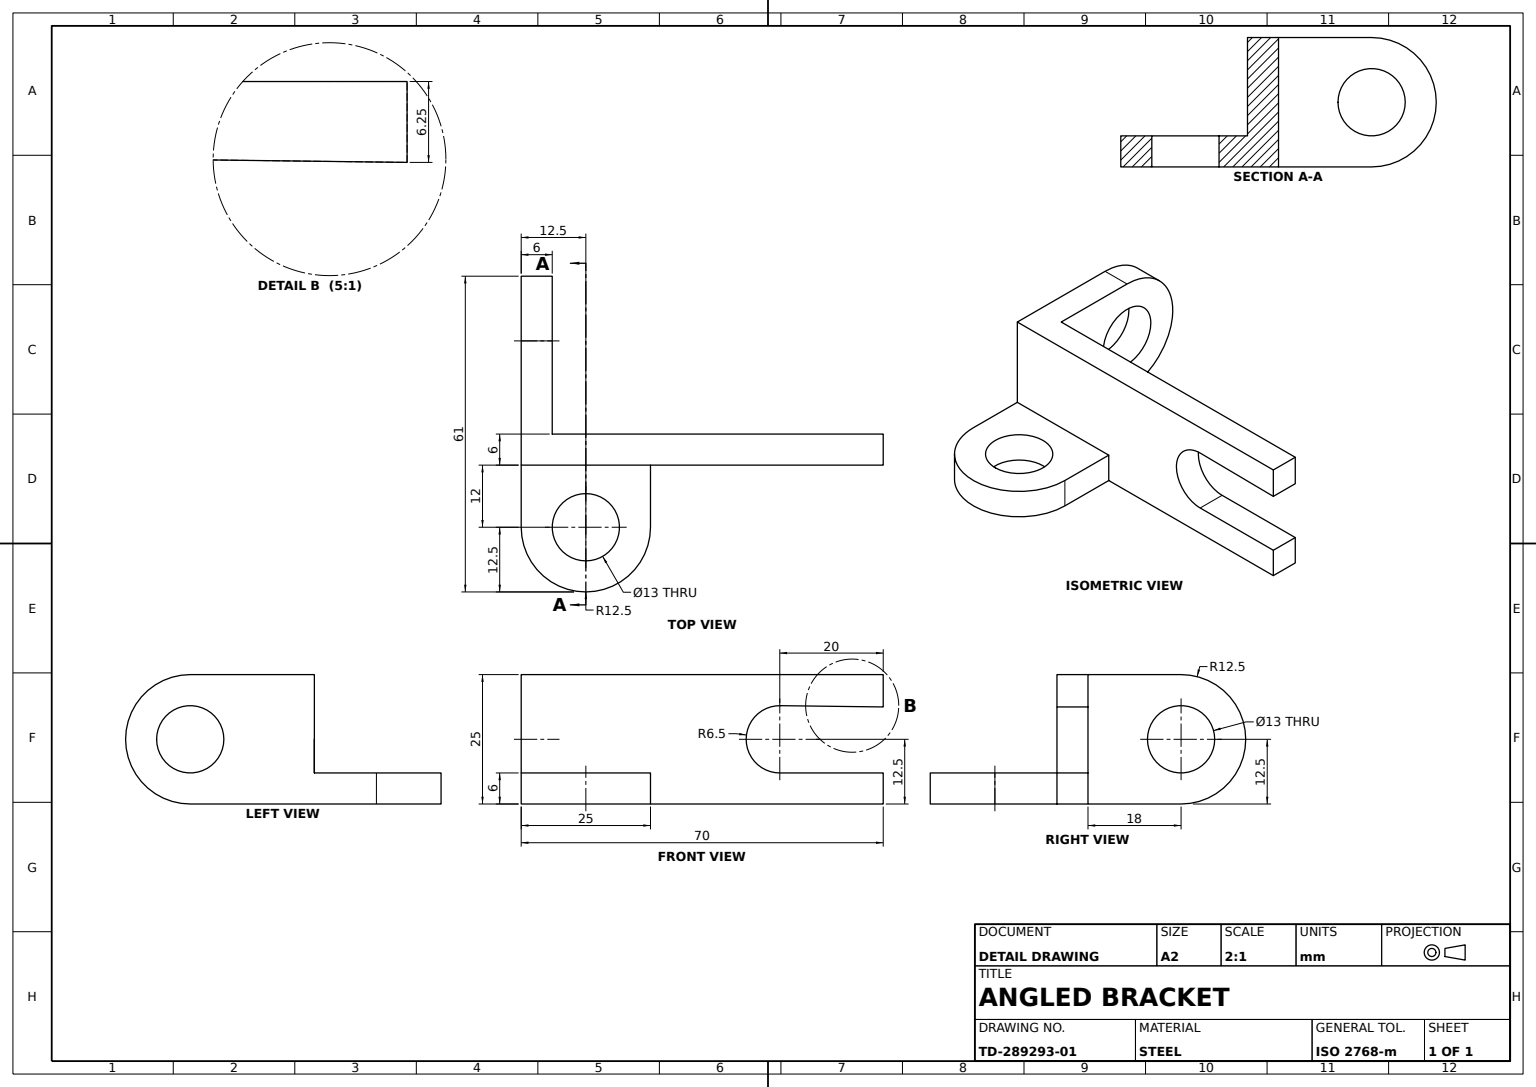
SolidWorks part; units mm, degrees
material "Plain Carbon Steel"
ref_plane "Front Plane" through (0, 0, 0) normal (0, 0, 1) x (1, 0, 0)
ref_plane "Top Plane" through (0, 0, 0) normal (0, 1, 0) x (1, 0, 0)
ref_plane "Right Plane" through (0, 0, 0) normal (1, 0, 0) x (0, 0, -1)
sketch "Bracket Profile Sketch" plane through (0, 0, 0) normal (0, 0, 1) x (1, 0, 0)
  line L0 (-35.4406, 0) -> (34.5594, 0)
  line L1 (-35.4406, 0) -> (-35.4406, 25)
  line L2 (-35.4406, 25) -> (34.5594, 25)
  line L3 (14.5594, 6) -> (34.5594, 6)
  line L4 (34.5594, 6) -> (34.5594, 0)
  line L5 (14.5594, 19) -> (34.5594, 18.75)
  line L6 (34.5594, 18.75) -> (34.5594, 25)
  arc A0 (14.7219, 18.998) -> (14.5594, 6) centre (14.5594, 12.5) ccw
  dimension "D5" = 13
  dimension "D1" = 25
  dimension "D2" = 70
  dimension "D3" = 70
  dimension "D4" = 35.4406
  dimension "D6" = 20
  dimension "D7" = 6
  dimension "D8" = 6.25
extrude "Slotted Bracket Body" add sketch "Bracket Profile Sketch" along normal blind 6 contours A0 L5 L6 L2 L1 L0 L4 L3
sketch "Lug A Sketch" plane through (-35.4406, 0, 0) normal (-1, 0, 0) x (0, 0, 1)
  line L1 (0, 0) -> (0, 25) construction
  line L2 (-18, 0) -> (6, 0)
  line L3 (6, 0) -> (6, 25)
  line L4 (6, 25) -> (-18, 25)
  arc A0 (-18, 25) -> (-18, 0) centre (-18, 12.5) ccw
  circle A1 centre (-18, 12.5) radius 6.5
  dimension "D2" = 25
  dimension "D3" = 18
  dimension "D1" = 13
extrude "Mounting Lug A Ø13" add sketch "Lug A Sketch" against normal blind 6
sketch "Lug B Sketch" plane through (0, 0, 0) normal (0, -1, 0) x (1, 0, 0)
  line L0 (-35.4406, 18) -> (-35.4406, 0)
  line L2 (-35.4406, 6) -> (-35.4406, -18) construction
  line L4 (-35.4406, 0) -> (-10.4406, 0)
  line L5 (-29.4406, 0) -> (34.5594, 0) construction
  line L6 (-10.4406, 0) -> (-10.4406, 18)
  arc A0 (-10.4406, 18) -> (-35.4406, 18) centre (-22.9406, 18) ccw
  circle A1 centre (-22.9406, 18) radius 6.5
  dimension "D3" = 25
  dimension "D1" = 13
  dimension "D2" = 12
extrude "Mounting Lug B Ø13" add sketch "Lug B Sketch" against normal blind 6
